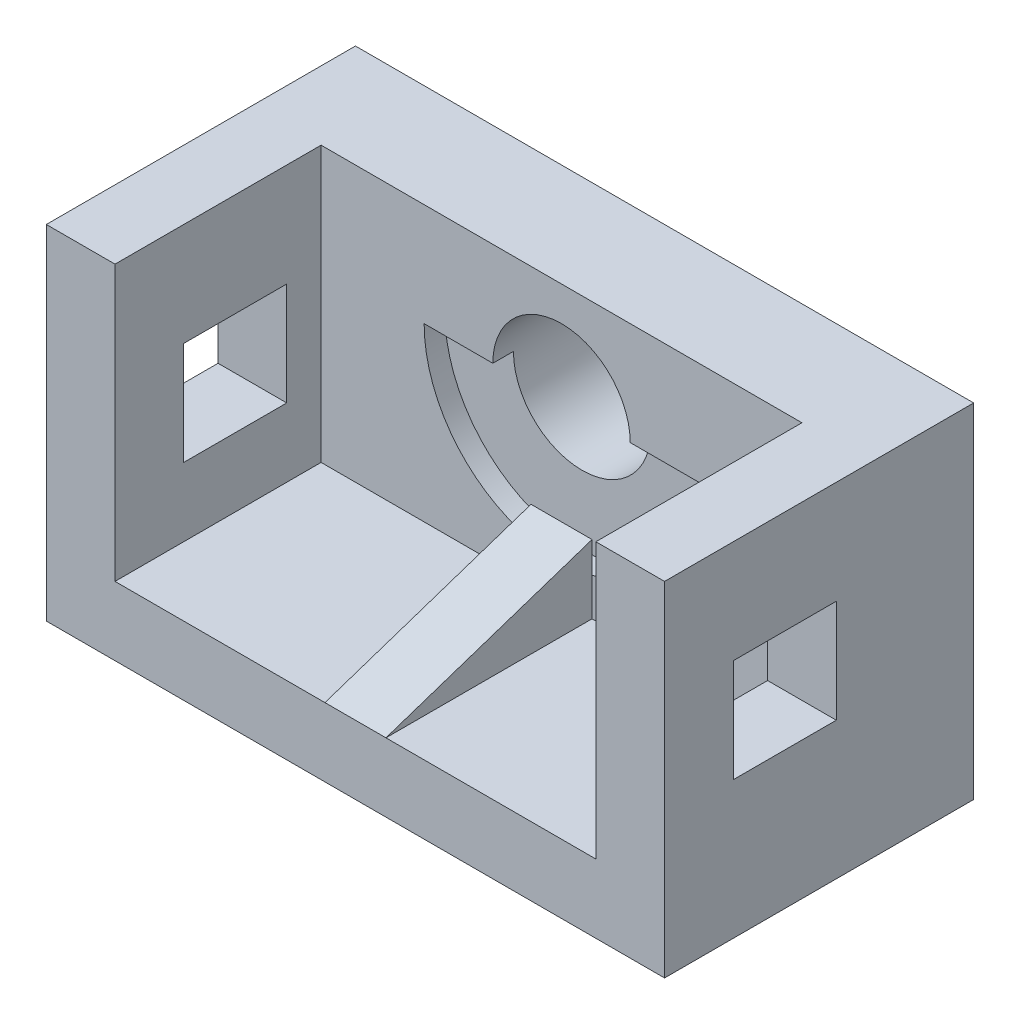
ISO-10303-21;
HEADER;
FILE_DESCRIPTION(('STEP AP214'),'2;1');
FILE_NAME('part.step','',(''),(''),'','','');
FILE_SCHEMA(('AUTOMOTIVE_DESIGN { 1 0 10303 214 1 1 1 1 }'));
ENDSEC;
DATA;
#1=APPLICATION_CONTEXT('core data for automotive mechanical design processes');
#2=APPLICATION_PROTOCOL_DEFINITION('international standard','automotive_design',2000,#1);
#3=PRODUCT_CONTEXT('',#1,'mechanical');
#4=PRODUCT('Part','Part','',(#3));
#5=PRODUCT_RELATED_PRODUCT_CATEGORY('part','',(#4));
#6=PRODUCT_DEFINITION_FORMATION('','',#4);
#7=PRODUCT_DEFINITION_CONTEXT('part definition',#1,'design');
#8=PRODUCT_DEFINITION('design','',#6,#7);
#9=PRODUCT_DEFINITION_SHAPE('','',#8);
#10=(LENGTH_UNIT() NAMED_UNIT(*) SI_UNIT(.MILLI.,.METRE.));
#11=(NAMED_UNIT(*) PLANE_ANGLE_UNIT() SI_UNIT($,.RADIAN.));
#12=(NAMED_UNIT(*) SI_UNIT($,.STERADIAN.) SOLID_ANGLE_UNIT());
#13=UNCERTAINTY_MEASURE_WITH_UNIT(LENGTH_MEASURE(1.E-05),#10,'distance_accuracy_value','');
#14=(GEOMETRIC_REPRESENTATION_CONTEXT(3) GLOBAL_UNCERTAINTY_ASSIGNED_CONTEXT((#13)) GLOBAL_UNIT_ASSIGNED_CONTEXT((#10,
#11,#12)) REPRESENTATION_CONTEXT('',''));
#15=CARTESIAN_POINT('',(0.,0.,0.));
#16=DIRECTION('',(0.,0.,1.));
#17=DIRECTION('',(1.,0.,0.));
#18=AXIS2_PLACEMENT_3D('',#15,#16,#17);
#19=CARTESIAN_POINT('',(-35.,-15.,-30.));
#20=DIRECTION('',(0.,-1.,0.));
#21=DIRECTION('',(0.,0.,-1.));
#22=AXIS2_PLACEMENT_3D('',#19,#20,#21);
#23=PLANE('',#22);
#24=DIRECTION('',(0.,0.,-1.));
#25=VECTOR('',#24,1.);
#26=CARTESIAN_POINT('',(-4.44066466837967,-15.,0.));
#27=LINE('',#26,#25);
#28=CARTESIAN_POINT('',(-4.44066466837967,-15.,0.));
#29=VERTEX_POINT('',#28);
#30=CARTESIAN_POINT('',(-4.44066466837967,-15.,-30.));
#31=VERTEX_POINT('',#30);
#32=EDGE_CURVE('E229',#29,#31,#27,.T.);
#33=ORIENTED_EDGE('',*,*,#32,.T.);
#34=DIRECTION('',(1.,0.,0.));
#35=VECTOR('',#34,1.);
#36=CARTESIAN_POINT('',(-35.,-15.,-30.));
#37=LINE('',#36,#35);
#38=CARTESIAN_POINT('',(-35.,-15.,-30.));
#39=VERTEX_POINT('',#38);
#40=EDGE_CURVE('E350',#39,#31,#37,.T.);
#41=ORIENTED_EDGE('',*,*,#40,.F.);
#42=DIRECTION('',(0.,0.,1.));
#43=VECTOR('',#42,1.);
#44=CARTESIAN_POINT('',(-35.,-15.,-30.));
#45=LINE('',#44,#43);
#46=CARTESIAN_POINT('',(-35.,-15.,0.));
#47=VERTEX_POINT('',#46);
#48=EDGE_CURVE('E254',#39,#47,#45,.T.);
#49=ORIENTED_EDGE('',*,*,#48,.T.);
#50=DIRECTION('',(1.,0.,0.));
#51=VECTOR('',#50,1.);
#52=CARTESIAN_POINT('',(-35.,-15.,0.));
#53=LINE('',#52,#51);
#54=EDGE_CURVE('E240',#47,#29,#53,.T.);
#55=ORIENTED_EDGE('',*,*,#54,.T.);
#56=EDGE_LOOP('',(#33,#41,#49,#55));
#57=FACE_BOUND('',#56,.T.);
#58=ADVANCED_FACE('F39',(#57),#23,.F.);
#59=DIRECTION('',(0.,0.,-1.));
#60=VECTOR('',#59,1.);
#61=CARTESIAN_POINT('',(4.44066466837967,-15.,0.));
#62=LINE('',#61,#60);
#63=CARTESIAN_POINT('',(4.44066466837967,-15.,0.));
#64=VERTEX_POINT('',#63);
#65=CARTESIAN_POINT('',(4.44066466837967,-15.,-30.));
#66=VERTEX_POINT('',#65);
#67=EDGE_CURVE('E218',#64,#66,#62,.T.);
#68=ORIENTED_EDGE('',*,*,#67,.F.);
#69=CARTESIAN_POINT('',(35.,-15.,0.));
#70=VERTEX_POINT('',#69);
#71=EDGE_CURVE('E227',#64,#70,#53,.T.);
#72=ORIENTED_EDGE('',*,*,#71,.T.);
#73=DIRECTION('',(0.,0.,1.));
#74=VECTOR('',#73,1.);
#75=CARTESIAN_POINT('',(35.,-15.,-30.));
#76=LINE('',#75,#74);
#77=CARTESIAN_POINT('',(35.,-15.,-30.));
#78=VERTEX_POINT('',#77);
#79=EDGE_CURVE('E252',#78,#70,#76,.T.);
#80=ORIENTED_EDGE('',*,*,#79,.F.);
#81=EDGE_CURVE('E230',#66,#78,#37,.T.);
#82=ORIENTED_EDGE('',*,*,#81,.F.);
#83=EDGE_LOOP('',(#68,#72,#80,#82));
#84=FACE_BOUND('',#83,.T.);
#85=ADVANCED_FACE('F222',(#84),#23,.F.);
#86=CARTESIAN_POINT('',(0.,0.,-30.));
#87=DIRECTION('',(0.,0.,1.));
#88=DIRECTION('',(1.,0.,0.));
#89=AXIS2_PLACEMENT_3D('',#86,#87,#88);
#90=PLANE('',#89);
#91=CARTESIAN_POINT('',(0.,10.,-30.));
#92=DIRECTION('',(0.,0.,1.));
#93=DIRECTION('',(1.,0.,0.));
#94=AXIS2_PLACEMENT_3D('',#91,#92,#93);
#95=CIRCLE('',#94,20.);
#96=CARTESIAN_POINT('',(-20.,10.,-30.));
#97=VERTEX_POINT('',#96);
#98=CARTESIAN_POINT('',(-4.44066466837967,-9.50078196644956,-30.));
#99=VERTEX_POINT('',#98);
#100=EDGE_CURVE('E371',#97,#99,#95,.T.);
#101=ORIENTED_EDGE('',*,*,#100,.F.);
#102=DIRECTION('',(-1.,0.,0.));
#103=VECTOR('',#102,1.);
#104=CARTESIAN_POINT('',(-10.,10.,-30.));
#105=LINE('',#104,#103);
#106=CARTESIAN_POINT('',(-10.,10.,-30.));
#107=VERTEX_POINT('',#106);
#108=EDGE_CURVE('E678',#107,#97,#105,.T.);
#109=ORIENTED_EDGE('',*,*,#108,.F.);
#110=CARTESIAN_POINT('',(0.,10.,-30.));
#111=DIRECTION('',(0.,0.,1.));
#112=DIRECTION('',(1.,0.,0.));
#113=AXIS2_PLACEMENT_3D('',#110,#111,#112);
#114=CIRCLE('',#113,10.);
#115=CARTESIAN_POINT('',(10.,10.,-30.));
#116=VERTEX_POINT('',#115);
#117=EDGE_CURVE('E336',#116,#107,#114,.T.);
#118=ORIENTED_EDGE('',*,*,#117,.F.);
#119=DIRECTION('',(-1.,0.,0.));
#120=VECTOR('',#119,1.);
#121=CARTESIAN_POINT('',(20.,10.,-30.));
#122=LINE('',#121,#120);
#123=CARTESIAN_POINT('',(20.,10.,-30.));
#124=VERTEX_POINT('',#123);
#125=EDGE_CURVE('E672',#124,#116,#122,.T.);
#126=ORIENTED_EDGE('',*,*,#125,.F.);
#127=CARTESIAN_POINT('',(4.44066466837967,-9.50078196644956,-30.));
#128=VERTEX_POINT('',#127);
#129=EDGE_CURVE('E668',#128,#124,#95,.T.);
#130=ORIENTED_EDGE('',*,*,#129,.F.);
#131=DIRECTION('',(0.,1.,0.));
#132=VECTOR('',#131,1.);
#133=CARTESIAN_POINT('',(4.44066466837967,-5.,-30.));
#134=LINE('',#133,#132);
#135=EDGE_CURVE('E377',#66,#128,#134,.T.);
#136=ORIENTED_EDGE('',*,*,#135,.F.);
#137=ORIENTED_EDGE('',*,*,#81,.T.);
#138=DIRECTION('',(0.,1.,0.));
#139=VECTOR('',#138,1.);
#140=CARTESIAN_POINT('',(35.,-15.,-30.));
#141=LINE('',#140,#139);
#142=CARTESIAN_POINT('',(35.,25.,-30.));
#143=VERTEX_POINT('',#142);
#144=EDGE_CURVE('E260',#78,#143,#141,.T.);
#145=ORIENTED_EDGE('',*,*,#144,.T.);
#146=DIRECTION('',(-1.,0.,0.));
#147=VECTOR('',#146,1.);
#148=CARTESIAN_POINT('',(35.,25.,-30.));
#149=LINE('',#148,#147);
#150=CARTESIAN_POINT('',(-35.,25.,-30.));
#151=VERTEX_POINT('',#150);
#152=EDGE_CURVE('E246',#143,#151,#149,.T.);
#153=ORIENTED_EDGE('',*,*,#152,.T.);
#154=DIRECTION('',(0.,-1.,0.));
#155=VECTOR('',#154,1.);
#156=CARTESIAN_POINT('',(-35.,25.,-30.));
#157=LINE('',#156,#155);
#158=EDGE_CURVE('E343',#151,#39,#157,.T.);
#159=ORIENTED_EDGE('',*,*,#158,.T.);
#160=ORIENTED_EDGE('',*,*,#40,.T.);
#161=DIRECTION('',(0.,-1.,0.));
#162=VECTOR('',#161,1.);
#163=CARTESIAN_POINT('',(-4.44066466837967,-5.,-30.));
#164=LINE('',#163,#162);
#165=EDGE_CURVE('E370',#99,#31,#164,.T.);
#166=ORIENTED_EDGE('',*,*,#165,.F.);
#167=EDGE_LOOP('',(#101,#109,#118,#126,#130,#136,#137,#145,#153,#159,#160,#166));
#168=FACE_BOUND('',#167,.T.);
#169=ADVANCED_FACE('F352',(#168),#90,.T.);
#170=CARTESIAN_POINT('',(45.,25.,-45.));
#171=DIRECTION('',(1.,0.,0.));
#172=DIRECTION('',(0.,0.,-1.));
#173=AXIS2_PLACEMENT_3D('',#170,#171,#172);
#174=PLANE('',#173);
#175=DIRECTION('',(0.,0.,1.));
#176=VECTOR('',#175,1.);
#177=CARTESIAN_POINT('',(45.,-5.,-10.));
#178=LINE('',#177,#176);
#179=CARTESIAN_POINT('',(45.,-5.,-25.));
#180=VERTEX_POINT('',#179);
#181=CARTESIAN_POINT('',(45.,-5.,-10.));
#182=VERTEX_POINT('',#181);
#183=EDGE_CURVE('E383',#180,#182,#178,.T.);
#184=ORIENTED_EDGE('',*,*,#183,.T.);
#185=DIRECTION('',(0.,1.,0.));
#186=VECTOR('',#185,1.);
#187=CARTESIAN_POINT('',(45.,10.,-10.));
#188=LINE('',#187,#186);
#189=CARTESIAN_POINT('',(45.,10.,-10.));
#190=VERTEX_POINT('',#189);
#191=EDGE_CURVE('E389',#182,#190,#188,.T.);
#192=ORIENTED_EDGE('',*,*,#191,.T.);
#193=DIRECTION('',(0.,0.,-1.));
#194=VECTOR('',#193,1.);
#195=CARTESIAN_POINT('',(45.,10.,-25.));
#196=LINE('',#195,#194);
#197=CARTESIAN_POINT('',(45.,10.,-25.));
#198=VERTEX_POINT('',#197);
#199=EDGE_CURVE('E53',#190,#198,#196,.T.);
#200=ORIENTED_EDGE('',*,*,#199,.T.);
#201=DIRECTION('',(0.,-1.,0.));
#202=VECTOR('',#201,1.);
#203=CARTESIAN_POINT('',(45.,-5.,-25.));
#204=LINE('',#203,#202);
#205=EDGE_CURVE('E395',#198,#180,#204,.T.);
#206=ORIENTED_EDGE('',*,*,#205,.T.);
#207=EDGE_LOOP('',(#184,#192,#200,#206));
#208=FACE_BOUND('',#207,.T.);
#209=DIRECTION('',(0.,1.,0.));
#210=VECTOR('',#209,1.);
#211=CARTESIAN_POINT('',(45.,25.,0.));
#212=LINE('',#211,#210);
#213=CARTESIAN_POINT('',(45.,-25.,0.));
#214=VERTEX_POINT('',#213);
#215=CARTESIAN_POINT('',(45.,25.,0.));
#216=VERTEX_POINT('',#215);
#217=EDGE_CURVE('E249',#214,#216,#212,.T.);
#218=ORIENTED_EDGE('',*,*,#217,.F.);
#219=DIRECTION('',(0.,0.,1.));
#220=VECTOR('',#219,1.);
#221=CARTESIAN_POINT('',(45.,-25.,-45.));
#222=LINE('',#221,#220);
#223=CARTESIAN_POINT('',(45.,-25.,-45.));
#224=VERTEX_POINT('',#223);
#225=EDGE_CURVE('E281',#224,#214,#222,.T.);
#226=ORIENTED_EDGE('',*,*,#225,.F.);
#227=DIRECTION('',(0.,1.,0.));
#228=VECTOR('',#227,1.);
#229=CARTESIAN_POINT('',(45.,25.,-45.));
#230=LINE('',#229,#228);
#231=CARTESIAN_POINT('',(45.,25.,-45.));
#232=VERTEX_POINT('',#231);
#233=EDGE_CURVE('E259',#224,#232,#230,.T.);
#234=ORIENTED_EDGE('',*,*,#233,.T.);
#235=DIRECTION('',(0.,0.,1.));
#236=VECTOR('',#235,1.);
#237=CARTESIAN_POINT('',(45.,25.,-45.));
#238=LINE('',#237,#236);
#239=EDGE_CURVE('E272',#232,#216,#238,.T.);
#240=ORIENTED_EDGE('',*,*,#239,.T.);
#241=EDGE_LOOP('',(#218,#226,#234,#240));
#242=FACE_BOUND('',#241,.T.);
#243=ADVANCED_FACE('F41',(#208,#242),#174,.T.);
#244=CARTESIAN_POINT('',(-45.,-25.,-45.));
#245=DIRECTION('',(0.,-1.,0.));
#246=DIRECTION('',(0.,0.,-1.));
#247=AXIS2_PLACEMENT_3D('',#244,#245,#246);
#248=PLANE('',#247);
#249=DIRECTION('',(1.,0.,0.));
#250=VECTOR('',#249,1.);
#251=CARTESIAN_POINT('',(-45.,-25.,0.));
#252=LINE('',#251,#250);
#253=CARTESIAN_POINT('',(-45.,-25.,0.));
#254=VERTEX_POINT('',#253);
#255=EDGE_CURVE('E261',#254,#214,#252,.T.);
#256=ORIENTED_EDGE('',*,*,#255,.F.);
#257=DIRECTION('',(0.,0.,1.));
#258=VECTOR('',#257,1.);
#259=CARTESIAN_POINT('',(-45.,-25.,-45.));
#260=LINE('',#259,#258);
#261=CARTESIAN_POINT('',(-45.,-25.,-45.));
#262=VERTEX_POINT('',#261);
#263=EDGE_CURVE('E282',#262,#254,#260,.T.);
#264=ORIENTED_EDGE('',*,*,#263,.F.);
#265=DIRECTION('',(1.,0.,0.));
#266=VECTOR('',#265,1.);
#267=CARTESIAN_POINT('',(-45.,-25.,-45.));
#268=LINE('',#267,#266);
#269=EDGE_CURVE('E270',#262,#224,#268,.T.);
#270=ORIENTED_EDGE('',*,*,#269,.T.);
#271=ORIENTED_EDGE('',*,*,#225,.T.);
#272=EDGE_LOOP('',(#256,#264,#270,#271));
#273=FACE_BOUND('',#272,.T.);
#274=ADVANCED_FACE('F425',(#273),#248,.T.);
#275=CARTESIAN_POINT('',(-45.,25.,-45.));
#276=DIRECTION('',(-1.,0.,0.));
#277=DIRECTION('',(0.,0.,1.));
#278=AXIS2_PLACEMENT_3D('',#275,#276,#277);
#279=PLANE('',#278);
#280=DIRECTION('',(0.,0.,1.));
#281=VECTOR('',#280,1.);
#282=CARTESIAN_POINT('',(-45.,-5.,-10.));
#283=LINE('',#282,#281);
#284=CARTESIAN_POINT('',(-45.,-5.,-25.));
#285=VERTEX_POINT('',#284);
#286=CARTESIAN_POINT('',(-45.,-5.,-10.));
#287=VERTEX_POINT('',#286);
#288=EDGE_CURVE('E65',#285,#287,#283,.T.);
#289=ORIENTED_EDGE('',*,*,#288,.F.);
#290=DIRECTION('',(0.,-1.,0.));
#291=VECTOR('',#290,1.);
#292=CARTESIAN_POINT('',(-45.,-5.,-25.));
#293=LINE('',#292,#291);
#294=CARTESIAN_POINT('',(-45.,10.,-25.));
#295=VERTEX_POINT('',#294);
#296=EDGE_CURVE('E386',#295,#285,#293,.T.);
#297=ORIENTED_EDGE('',*,*,#296,.F.);
#298=DIRECTION('',(0.,0.,-1.));
#299=VECTOR('',#298,1.);
#300=CARTESIAN_POINT('',(-45.,10.,-25.));
#301=LINE('',#300,#299);
#302=CARTESIAN_POINT('',(-45.,10.,-10.));
#303=VERTEX_POINT('',#302);
#304=EDGE_CURVE('E311',#303,#295,#301,.T.);
#305=ORIENTED_EDGE('',*,*,#304,.F.);
#306=DIRECTION('',(0.,1.,0.));
#307=VECTOR('',#306,1.);
#308=CARTESIAN_POINT('',(-45.,10.,-10.));
#309=LINE('',#308,#307);
#310=EDGE_CURVE('E396',#287,#303,#309,.T.);
#311=ORIENTED_EDGE('',*,*,#310,.F.);
#312=EDGE_LOOP('',(#289,#297,#305,#311));
#313=FACE_BOUND('',#312,.T.);
#314=DIRECTION('',(0.,-1.,0.));
#315=VECTOR('',#314,1.);
#316=CARTESIAN_POINT('',(-45.,25.,0.));
#317=LINE('',#316,#315);
#318=CARTESIAN_POINT('',(-45.,25.,0.));
#319=VERTEX_POINT('',#318);
#320=EDGE_CURVE('E280',#319,#254,#317,.T.);
#321=ORIENTED_EDGE('',*,*,#320,.F.);
#322=DIRECTION('',(0.,0.,1.));
#323=VECTOR('',#322,1.);
#324=CARTESIAN_POINT('',(-45.,25.,-45.));
#325=LINE('',#324,#323);
#326=CARTESIAN_POINT('',(-45.,25.,-45.));
#327=VERTEX_POINT('',#326);
#328=EDGE_CURVE('E286',#327,#319,#325,.T.);
#329=ORIENTED_EDGE('',*,*,#328,.F.);
#330=DIRECTION('',(0.,-1.,0.));
#331=VECTOR('',#330,1.);
#332=CARTESIAN_POINT('',(-45.,25.,-45.));
#333=LINE('',#332,#331);
#334=EDGE_CURVE('E262',#327,#262,#333,.T.);
#335=ORIENTED_EDGE('',*,*,#334,.T.);
#336=ORIENTED_EDGE('',*,*,#263,.T.);
#337=EDGE_LOOP('',(#321,#329,#335,#336));
#338=FACE_BOUND('',#337,.T.);
#339=ADVANCED_FACE('F405',(#313,#338),#279,.T.);
#340=CARTESIAN_POINT('',(-45.,25.,-45.));
#341=DIRECTION('',(0.,1.,0.));
#342=DIRECTION('',(-1.,0.,0.));
#343=AXIS2_PLACEMENT_3D('',#340,#341,#342);
#344=PLANE('',#343);
#345=DIRECTION('',(0.,0.,1.));
#346=VECTOR('',#345,1.);
#347=CARTESIAN_POINT('',(35.,25.,-30.));
#348=LINE('',#347,#346);
#349=CARTESIAN_POINT('',(35.,25.,0.));
#350=VERTEX_POINT('',#349);
#351=EDGE_CURVE('E250',#143,#350,#348,.T.);
#352=ORIENTED_EDGE('',*,*,#351,.T.);
#353=DIRECTION('',(-1.,0.,0.));
#354=VECTOR('',#353,1.);
#355=CARTESIAN_POINT('',(-45.,25.,0.));
#356=LINE('',#355,#354);
#357=EDGE_CURVE('E273',#216,#350,#356,.T.);
#358=ORIENTED_EDGE('',*,*,#357,.F.);
#359=ORIENTED_EDGE('',*,*,#239,.F.);
#360=DIRECTION('',(-1.,0.,0.));
#361=VECTOR('',#360,1.);
#362=CARTESIAN_POINT('',(-45.,25.,-45.));
#363=LINE('',#362,#361);
#364=EDGE_CURVE('E264',#232,#327,#363,.T.);
#365=ORIENTED_EDGE('',*,*,#364,.T.);
#366=ORIENTED_EDGE('',*,*,#328,.T.);
#367=CARTESIAN_POINT('',(-35.,25.,0.));
#368=VERTEX_POINT('',#367);
#369=EDGE_CURVE('E274',#368,#319,#356,.T.);
#370=ORIENTED_EDGE('',*,*,#369,.F.);
#371=DIRECTION('',(0.,0.,1.));
#372=VECTOR('',#371,1.);
#373=CARTESIAN_POINT('',(-35.,25.,-30.));
#374=LINE('',#373,#372);
#375=EDGE_CURVE('E253',#151,#368,#374,.T.);
#376=ORIENTED_EDGE('',*,*,#375,.F.);
#377=ORIENTED_EDGE('',*,*,#152,.F.);
#378=EDGE_LOOP('',(#352,#358,#359,#365,#366,#370,#376,#377));
#379=FACE_BOUND('',#378,.T.);
#380=ADVANCED_FACE('F360',(#379),#344,.T.);
#381=CARTESIAN_POINT('',(0.,0.,-45.));
#382=DIRECTION('',(0.,0.,1.));
#383=DIRECTION('',(1.,0.,0.));
#384=AXIS2_PLACEMENT_3D('',#381,#382,#383);
#385=PLANE('',#384);
#386=CARTESIAN_POINT('',(0.,10.,-45.));
#387=DIRECTION('',(0.,0.,1.));
#388=DIRECTION('',(1.,0.,0.));
#389=AXIS2_PLACEMENT_3D('',#386,#387,#388);
#390=CIRCLE('',#389,10.);
#391=CARTESIAN_POINT('',(10.,10.,-45.));
#392=VERTEX_POINT('',#391);
#393=EDGE_CURVE('E241',#392,#392,#390,.T.);
#394=ORIENTED_EDGE('',*,*,#393,.T.);
#395=EDGE_LOOP('',(#394));
#396=FACE_BOUND('',#395,.T.);
#397=ORIENTED_EDGE('',*,*,#233,.F.);
#398=ORIENTED_EDGE('',*,*,#269,.F.);
#399=ORIENTED_EDGE('',*,*,#334,.F.);
#400=ORIENTED_EDGE('',*,*,#364,.F.);
#401=EDGE_LOOP('',(#397,#398,#399,#400));
#402=FACE_BOUND('',#401,.T.);
#403=ADVANCED_FACE('F433',(#396,#402),#385,.F.);
#404=CARTESIAN_POINT('',(0.,0.,0.));
#405=DIRECTION('',(0.,0.,1.));
#406=DIRECTION('',(1.,0.,0.));
#407=AXIS2_PLACEMENT_3D('',#404,#405,#406);
#408=PLANE('',#407);
#409=DIRECTION('',(1.,0.,0.));
#410=VECTOR('',#409,1.);
#411=CARTESIAN_POINT('',(-5.55933533162033,-15.,0.));
#412=LINE('',#411,#410);
#413=EDGE_CURVE('E201',#29,#64,#412,.T.);
#414=ORIENTED_EDGE('',*,*,#413,.F.);
#415=ORIENTED_EDGE('',*,*,#54,.F.);
#416=DIRECTION('',(0.,-1.,0.));
#417=VECTOR('',#416,1.);
#418=CARTESIAN_POINT('',(-35.,25.,0.));
#419=LINE('',#418,#417);
#420=EDGE_CURVE('E238',#368,#47,#419,.T.);
#421=ORIENTED_EDGE('',*,*,#420,.F.);
#422=ORIENTED_EDGE('',*,*,#369,.T.);
#423=ORIENTED_EDGE('',*,*,#320,.T.);
#424=ORIENTED_EDGE('',*,*,#255,.T.);
#425=ORIENTED_EDGE('',*,*,#217,.T.);
#426=ORIENTED_EDGE('',*,*,#357,.T.);
#427=DIRECTION('',(0.,1.,0.));
#428=VECTOR('',#427,1.);
#429=CARTESIAN_POINT('',(35.,-15.,0.));
#430=LINE('',#429,#428);
#431=EDGE_CURVE('E236',#70,#350,#430,.T.);
#432=ORIENTED_EDGE('',*,*,#431,.F.);
#433=ORIENTED_EDGE('',*,*,#71,.F.);
#434=EDGE_LOOP('',(#414,#415,#421,#422,#423,#424,#425,#426,#432,#433));
#435=FACE_BOUND('',#434,.T.);
#436=ADVANCED_FACE('F234',(#435),#408,.T.);
#437=CARTESIAN_POINT('',(35.,-15.,-30.));
#438=DIRECTION('',(1.,0.,0.));
#439=DIRECTION('',(0.,1.,0.));
#440=AXIS2_PLACEMENT_3D('',#437,#438,#439);
#441=PLANE('',#440);
#442=DIRECTION('',(0.,-1.,0.));
#443=VECTOR('',#442,1.);
#444=CARTESIAN_POINT('',(35.,-15.,-10.));
#445=LINE('',#444,#443);
#446=CARTESIAN_POINT('',(35.,10.,-10.));
#447=VERTEX_POINT('',#446);
#448=CARTESIAN_POINT('',(35.,-5.,-10.));
#449=VERTEX_POINT('',#448);
#450=EDGE_CURVE('E329',#447,#449,#445,.T.);
#451=ORIENTED_EDGE('',*,*,#450,.T.);
#452=DIRECTION('',(0.,0.,-1.));
#453=VECTOR('',#452,1.);
#454=CARTESIAN_POINT('',(35.,-5.,-30.));
#455=LINE('',#454,#453);
#456=CARTESIAN_POINT('',(35.,-5.,-25.));
#457=VERTEX_POINT('',#456);
#458=EDGE_CURVE('E332',#449,#457,#455,.T.);
#459=ORIENTED_EDGE('',*,*,#458,.T.);
#460=DIRECTION('',(0.,1.,0.));
#461=VECTOR('',#460,1.);
#462=CARTESIAN_POINT('',(35.,-15.,-25.));
#463=LINE('',#462,#461);
#464=CARTESIAN_POINT('',(35.,10.,-25.));
#465=VERTEX_POINT('',#464);
#466=EDGE_CURVE('E331',#457,#465,#463,.T.);
#467=ORIENTED_EDGE('',*,*,#466,.T.);
#468=DIRECTION('',(0.,0.,1.));
#469=VECTOR('',#468,1.);
#470=CARTESIAN_POINT('',(35.,10.,-30.));
#471=LINE('',#470,#469);
#472=EDGE_CURVE('E328',#465,#447,#471,.T.);
#473=ORIENTED_EDGE('',*,*,#472,.T.);
#474=EDGE_LOOP('',(#451,#459,#467,#473));
#475=FACE_BOUND('',#474,.T.);
#476=ORIENTED_EDGE('',*,*,#431,.T.);
#477=ORIENTED_EDGE('',*,*,#351,.F.);
#478=ORIENTED_EDGE('',*,*,#144,.F.);
#479=ORIENTED_EDGE('',*,*,#79,.T.);
#480=EDGE_LOOP('',(#476,#477,#478,#479));
#481=FACE_BOUND('',#480,.T.);
#482=ADVANCED_FACE('F412',(#475,#481),#441,.F.);
#483=CARTESIAN_POINT('',(-35.,25.,-30.));
#484=DIRECTION('',(-1.,0.,0.));
#485=DIRECTION('',(0.,-1.,0.));
#486=AXIS2_PLACEMENT_3D('',#483,#484,#485);
#487=PLANE('',#486);
#488=DIRECTION('',(0.,-1.,0.));
#489=VECTOR('',#488,1.);
#490=CARTESIAN_POINT('',(-35.,25.,-25.));
#491=LINE('',#490,#489);
#492=CARTESIAN_POINT('',(-35.,10.,-25.));
#493=VERTEX_POINT('',#492);
#494=CARTESIAN_POINT('',(-35.,-5.,-25.));
#495=VERTEX_POINT('',#494);
#496=EDGE_CURVE('E50',#493,#495,#491,.T.);
#497=ORIENTED_EDGE('',*,*,#496,.T.);
#498=DIRECTION('',(0.,0.,1.));
#499=VECTOR('',#498,1.);
#500=CARTESIAN_POINT('',(-35.,-5.,-30.));
#501=LINE('',#500,#499);
#502=CARTESIAN_POINT('',(-35.,-5.,-10.));
#503=VERTEX_POINT('',#502);
#504=EDGE_CURVE('E11',#495,#503,#501,.T.);
#505=ORIENTED_EDGE('',*,*,#504,.T.);
#506=DIRECTION('',(0.,1.,0.));
#507=VECTOR('',#506,1.);
#508=CARTESIAN_POINT('',(-35.,25.,-10.));
#509=LINE('',#508,#507);
#510=CARTESIAN_POINT('',(-35.,10.,-10.));
#511=VERTEX_POINT('',#510);
#512=EDGE_CURVE('E283',#503,#511,#509,.T.);
#513=ORIENTED_EDGE('',*,*,#512,.T.);
#514=DIRECTION('',(0.,0.,-1.));
#515=VECTOR('',#514,1.);
#516=CARTESIAN_POINT('',(-35.,10.,-30.));
#517=LINE('',#516,#515);
#518=EDGE_CURVE('E291',#511,#493,#517,.T.);
#519=ORIENTED_EDGE('',*,*,#518,.T.);
#520=EDGE_LOOP('',(#497,#505,#513,#519));
#521=FACE_BOUND('',#520,.T.);
#522=ORIENTED_EDGE('',*,*,#420,.T.);
#523=ORIENTED_EDGE('',*,*,#48,.F.);
#524=ORIENTED_EDGE('',*,*,#158,.F.);
#525=ORIENTED_EDGE('',*,*,#375,.T.);
#526=EDGE_LOOP('',(#522,#523,#524,#525));
#527=FACE_BOUND('',#526,.T.);
#528=ADVANCED_FACE('F300',(#521,#527),#487,.F.);
#529=CARTESIAN_POINT('',(0.,10.,-45.));
#530=DIRECTION('',(0.,0.,1.));
#531=DIRECTION('',(1.,0.,0.));
#532=AXIS2_PLACEMENT_3D('',#529,#530,#531);
#533=CYLINDRICAL_SURFACE('',#532,10.);
#534=ORIENTED_EDGE('',*,*,#117,.T.);
#535=DIRECTION('',(0.,0.,1.));
#536=VECTOR('',#535,1.);
#537=CARTESIAN_POINT('',(-10.,10.,-33.));
#538=LINE('',#537,#536);
#539=CARTESIAN_POINT('',(-10.,10.,-33.));
#540=VERTEX_POINT('',#539);
#541=EDGE_CURVE('E688',#540,#107,#538,.T.);
#542=ORIENTED_EDGE('',*,*,#541,.F.);
#543=CARTESIAN_POINT('',(0.,10.,-33.));
#544=DIRECTION('',(0.,0.,-1.));
#545=DIRECTION('',(1.,0.,0.));
#546=AXIS2_PLACEMENT_3D('',#543,#544,#545);
#547=CIRCLE('',#546,10.);
#548=CARTESIAN_POINT('',(10.,10.,-33.));
#549=VERTEX_POINT('',#548);
#550=EDGE_CURVE('E693',#549,#540,#547,.T.);
#551=ORIENTED_EDGE('',*,*,#550,.F.);
#552=DIRECTION('',(0.,0.,1.));
#553=VECTOR('',#552,1.);
#554=CARTESIAN_POINT('',(10.,10.,-33.));
#555=LINE('',#554,#553);
#556=EDGE_CURVE('E686',#549,#116,#555,.T.);
#557=ORIENTED_EDGE('',*,*,#556,.T.);
#558=EDGE_LOOP('',(#534,#542,#551,#557));
#559=FACE_BOUND('',#558,.T.);
#560=ORIENTED_EDGE('',*,*,#393,.F.);
#561=EDGE_LOOP('',(#560));
#562=FACE_BOUND('',#561,.T.);
#563=ADVANCED_FACE('F451',(#559,#562),#533,.F.);
#564=CARTESIAN_POINT('',(45.,10.,-10.));
#565=DIRECTION('',(0.,0.,1.));
#566=DIRECTION('',(1.,0.,0.));
#567=AXIS2_PLACEMENT_3D('',#564,#565,#566);
#568=PLANE('',#567);
#569=DIRECTION('',(-1.,0.,0.));
#570=VECTOR('',#569,1.);
#571=CARTESIAN_POINT('',(45.,-5.,-10.));
#572=LINE('',#571,#570);
#573=EDGE_CURVE('E323',#503,#287,#572,.T.);
#574=ORIENTED_EDGE('',*,*,#573,.T.);
#575=ORIENTED_EDGE('',*,*,#310,.T.);
#576=DIRECTION('',(-1.,0.,0.));
#577=VECTOR('',#576,1.);
#578=CARTESIAN_POINT('',(45.,10.,-10.));
#579=LINE('',#578,#577);
#580=EDGE_CURVE('E320',#511,#303,#579,.T.);
#581=ORIENTED_EDGE('',*,*,#580,.F.);
#582=ORIENTED_EDGE('',*,*,#512,.F.);
#583=EDGE_LOOP('',(#574,#575,#581,#582));
#584=FACE_BOUND('',#583,.T.);
#585=ADVANCED_FACE('F403',(#584),#568,.F.);
#586=CARTESIAN_POINT('',(45.,10.,-25.));
#587=DIRECTION('',(0.,1.,0.));
#588=DIRECTION('',(0.,0.,1.));
#589=AXIS2_PLACEMENT_3D('',#586,#587,#588);
#590=PLANE('',#589);
#591=ORIENTED_EDGE('',*,*,#580,.T.);
#592=ORIENTED_EDGE('',*,*,#304,.T.);
#593=DIRECTION('',(-1.,0.,0.));
#594=VECTOR('',#593,1.);
#595=CARTESIAN_POINT('',(45.,10.,-25.));
#596=LINE('',#595,#594);
#597=EDGE_CURVE('E304',#493,#295,#596,.T.);
#598=ORIENTED_EDGE('',*,*,#597,.F.);
#599=ORIENTED_EDGE('',*,*,#518,.F.);
#600=EDGE_LOOP('',(#591,#592,#598,#599));
#601=FACE_BOUND('',#600,.T.);
#602=ADVANCED_FACE('F307',(#601),#590,.F.);
#603=CARTESIAN_POINT('',(45.,-5.,-25.));
#604=DIRECTION('',(0.,0.,-1.));
#605=DIRECTION('',(-1.,0.,0.));
#606=AXIS2_PLACEMENT_3D('',#603,#604,#605);
#607=PLANE('',#606);
#608=ORIENTED_EDGE('',*,*,#597,.T.);
#609=ORIENTED_EDGE('',*,*,#296,.T.);
#610=DIRECTION('',(-1.,0.,0.));
#611=VECTOR('',#610,1.);
#612=CARTESIAN_POINT('',(45.,-5.,-25.));
#613=LINE('',#612,#611);
#614=EDGE_CURVE('E310',#495,#285,#613,.T.);
#615=ORIENTED_EDGE('',*,*,#614,.F.);
#616=ORIENTED_EDGE('',*,*,#496,.F.);
#617=EDGE_LOOP('',(#608,#609,#615,#616));
#618=FACE_BOUND('',#617,.T.);
#619=ADVANCED_FACE('F303',(#618),#607,.F.);
#620=CARTESIAN_POINT('',(45.,-5.,-10.));
#621=DIRECTION('',(0.,-1.,0.));
#622=DIRECTION('',(0.,0.,-1.));
#623=AXIS2_PLACEMENT_3D('',#620,#621,#622);
#624=PLANE('',#623);
#625=ORIENTED_EDGE('',*,*,#614,.T.);
#626=ORIENTED_EDGE('',*,*,#288,.T.);
#627=ORIENTED_EDGE('',*,*,#573,.F.);
#628=ORIENTED_EDGE('',*,*,#504,.F.);
#629=EDGE_LOOP('',(#625,#626,#627,#628));
#630=FACE_BOUND('',#629,.T.);
#631=ADVANCED_FACE('F407',(#630),#624,.F.);
#632=EDGE_CURVE('E324',#182,#449,#572,.T.);
#633=ORIENTED_EDGE('',*,*,#632,.F.);
#634=ORIENTED_EDGE('',*,*,#183,.F.);
#635=EDGE_CURVE('E318',#180,#457,#613,.T.);
#636=ORIENTED_EDGE('',*,*,#635,.T.);
#637=ORIENTED_EDGE('',*,*,#458,.F.);
#638=EDGE_LOOP('',(#633,#634,#636,#637));
#639=FACE_BOUND('',#638,.T.);
#640=ADVANCED_FACE('F414',(#639),#624,.F.);
#641=ORIENTED_EDGE('',*,*,#635,.F.);
#642=ORIENTED_EDGE('',*,*,#205,.F.);
#643=EDGE_CURVE('E312',#198,#465,#596,.T.);
#644=ORIENTED_EDGE('',*,*,#643,.T.);
#645=ORIENTED_EDGE('',*,*,#466,.F.);
#646=EDGE_LOOP('',(#641,#642,#644,#645));
#647=FACE_BOUND('',#646,.T.);
#648=ADVANCED_FACE('F417',(#647),#607,.F.);
#649=ORIENTED_EDGE('',*,*,#643,.F.);
#650=ORIENTED_EDGE('',*,*,#199,.F.);
#651=EDGE_CURVE('E313',#190,#447,#579,.T.);
#652=ORIENTED_EDGE('',*,*,#651,.T.);
#653=ORIENTED_EDGE('',*,*,#472,.F.);
#654=EDGE_LOOP('',(#649,#650,#652,#653));
#655=FACE_BOUND('',#654,.T.);
#656=ADVANCED_FACE('F418',(#655),#590,.F.);
#657=ORIENTED_EDGE('',*,*,#651,.F.);
#658=ORIENTED_EDGE('',*,*,#191,.F.);
#659=ORIENTED_EDGE('',*,*,#632,.T.);
#660=ORIENTED_EDGE('',*,*,#450,.F.);
#661=EDGE_LOOP('',(#657,#658,#659,#660));
#662=FACE_BOUND('',#661,.T.);
#663=ADVANCED_FACE('F416',(#662),#568,.F.);
#664=CARTESIAN_POINT('',(-4.44066466837967,-5.,0.));
#665=DIRECTION('',(1.,0.,0.));
#666=DIRECTION('',(0.,1.,0.));
#667=AXIS2_PLACEMENT_3D('',#664,#665,#666);
#668=PLANE('',#667);
#669=ORIENTED_EDGE('',*,*,#32,.F.);
#670=DIRECTION('',(0.,0.316227766016838,-0.948683298050514));
#671=VECTOR('',#670,1.);
#672=CARTESIAN_POINT('',(-4.44066466837967,-14.,-3.));
#673=LINE('',#672,#671);
#674=CARTESIAN_POINT('',(-4.44066466837967,-5.,-30.));
#675=VERTEX_POINT('',#674);
#676=EDGE_CURVE('E206',#29,#675,#673,.T.);
#677=ORIENTED_EDGE('',*,*,#676,.T.);
#678=EDGE_CURVE('E373',#675,#99,#164,.T.);
#679=ORIENTED_EDGE('',*,*,#678,.T.);
#680=ORIENTED_EDGE('',*,*,#165,.T.);
#681=EDGE_LOOP('',(#669,#677,#679,#680));
#682=FACE_BOUND('',#681,.T.);
#683=ADVANCED_FACE('F376',(#682),#668,.F.);
#684=CARTESIAN_POINT('',(4.44066466837967,-5.,0.));
#685=DIRECTION('',(-1.,0.,0.));
#686=DIRECTION('',(0.,-1.,0.));
#687=AXIS2_PLACEMENT_3D('',#684,#685,#686);
#688=PLANE('',#687);
#689=DIRECTION('',(0.,1.,0.));
#690=VECTOR('',#689,1.);
#691=CARTESIAN_POINT('',(4.44066466837967,-5.,-30.));
#692=LINE('',#691,#690);
#693=CARTESIAN_POINT('',(4.44066466837967,-5.,-30.));
#694=VERTEX_POINT('',#693);
#695=EDGE_CURVE('E224',#128,#694,#692,.T.);
#696=ORIENTED_EDGE('',*,*,#695,.T.);
#697=DIRECTION('',(0.,0.316227766016838,-0.948683298050514));
#698=VECTOR('',#697,1.);
#699=CARTESIAN_POINT('',(4.44066466837967,-15.,0.));
#700=LINE('',#699,#698);
#701=EDGE_CURVE('E202',#64,#694,#700,.T.);
#702=ORIENTED_EDGE('',*,*,#701,.F.);
#703=ORIENTED_EDGE('',*,*,#67,.T.);
#704=ORIENTED_EDGE('',*,*,#135,.T.);
#705=EDGE_LOOP('',(#696,#702,#703,#704));
#706=FACE_BOUND('',#705,.T.);
#707=ADVANCED_FACE('F216',(#706),#688,.F.);
#708=CARTESIAN_POINT('',(0.,10.,-30.));
#709=DIRECTION('',(0.,0.,1.));
#710=DIRECTION('',(1.,0.,0.));
#711=AXIS2_PLACEMENT_3D('',#708,#709,#710);
#712=PLANE('',#711);
#713=DIRECTION('',(-1.,0.,0.));
#714=VECTOR('',#713,1.);
#715=CARTESIAN_POINT('',(4.44066466837967,-5.,-30.));
#716=LINE('',#715,#714);
#717=EDGE_CURVE('E233',#694,#675,#716,.T.);
#718=ORIENTED_EDGE('',*,*,#717,.F.);
#719=ORIENTED_EDGE('',*,*,#695,.F.);
#720=EDGE_CURVE('E670',#99,#128,#95,.T.);
#721=ORIENTED_EDGE('',*,*,#720,.F.);
#722=ORIENTED_EDGE('',*,*,#678,.F.);
#723=EDGE_LOOP('',(#718,#719,#721,#722));
#724=FACE_BOUND('',#723,.T.);
#725=ADVANCED_FACE('F542',(#724),#712,.F.);
#726=CARTESIAN_POINT('',(0.,10.,-33.));
#727=DIRECTION('',(0.,0.,1.));
#728=DIRECTION('',(1.,0.,0.));
#729=AXIS2_PLACEMENT_3D('',#726,#727,#728);
#730=CYLINDRICAL_SURFACE('',#729,20.);
#731=ORIENTED_EDGE('',*,*,#100,.T.);
#732=ORIENTED_EDGE('',*,*,#720,.T.);
#733=ORIENTED_EDGE('',*,*,#129,.T.);
#734=DIRECTION('',(0.,0.,1.));
#735=VECTOR('',#734,1.);
#736=CARTESIAN_POINT('',(20.,10.,-33.));
#737=LINE('',#736,#735);
#738=CARTESIAN_POINT('',(20.,10.,-33.));
#739=VERTEX_POINT('',#738);
#740=EDGE_CURVE('E689',#739,#124,#737,.T.);
#741=ORIENTED_EDGE('',*,*,#740,.F.);
#742=CARTESIAN_POINT('',(0.,10.,-33.));
#743=DIRECTION('',(0.,0.,1.));
#744=DIRECTION('',(1.,0.,0.));
#745=AXIS2_PLACEMENT_3D('',#742,#743,#744);
#746=CIRCLE('',#745,20.);
#747=CARTESIAN_POINT('',(-20.,10.,-33.));
#748=VERTEX_POINT('',#747);
#749=EDGE_CURVE('E682',#748,#739,#746,.T.);
#750=ORIENTED_EDGE('',*,*,#749,.F.);
#751=DIRECTION('',(0.,0.,1.));
#752=VECTOR('',#751,1.);
#753=CARTESIAN_POINT('',(-20.,10.,-33.));
#754=LINE('',#753,#752);
#755=EDGE_CURVE('E669',#748,#97,#754,.T.);
#756=ORIENTED_EDGE('',*,*,#755,.T.);
#757=EDGE_LOOP('',(#731,#732,#733,#741,#750,#756));
#758=FACE_BOUND('',#757,.T.);
#759=ADVANCED_FACE('F538',(#758),#730,.F.);
#760=CARTESIAN_POINT('',(-10.,10.,-33.));
#761=DIRECTION('',(0.,1.,0.));
#762=DIRECTION('',(0.,0.,1.));
#763=AXIS2_PLACEMENT_3D('',#760,#761,#762);
#764=PLANE('',#763);
#765=ORIENTED_EDGE('',*,*,#108,.T.);
#766=ORIENTED_EDGE('',*,*,#755,.F.);
#767=DIRECTION('',(-1.,0.,0.));
#768=VECTOR('',#767,1.);
#769=CARTESIAN_POINT('',(-10.,10.,-33.));
#770=LINE('',#769,#768);
#771=EDGE_CURVE('E687',#540,#748,#770,.T.);
#772=ORIENTED_EDGE('',*,*,#771,.F.);
#773=ORIENTED_EDGE('',*,*,#541,.T.);
#774=EDGE_LOOP('',(#765,#766,#772,#773));
#775=FACE_BOUND('',#774,.T.);
#776=ADVANCED_FACE('F543',(#775),#764,.F.);
#777=CARTESIAN_POINT('',(20.,10.,-33.));
#778=DIRECTION('',(0.,1.,0.));
#779=DIRECTION('',(0.,0.,1.));
#780=AXIS2_PLACEMENT_3D('',#777,#778,#779);
#781=PLANE('',#780);
#782=ORIENTED_EDGE('',*,*,#125,.T.);
#783=ORIENTED_EDGE('',*,*,#556,.F.);
#784=DIRECTION('',(-1.,0.,0.));
#785=VECTOR('',#784,1.);
#786=CARTESIAN_POINT('',(20.,10.,-33.));
#787=LINE('',#786,#785);
#788=EDGE_CURVE('E696',#739,#549,#787,.T.);
#789=ORIENTED_EDGE('',*,*,#788,.F.);
#790=ORIENTED_EDGE('',*,*,#740,.T.);
#791=EDGE_LOOP('',(#782,#783,#789,#790));
#792=FACE_BOUND('',#791,.T.);
#793=ADVANCED_FACE('F554',(#792),#781,.F.);
#794=CARTESIAN_POINT('',(0.,10.,-33.));
#795=DIRECTION('',(0.,0.,1.));
#796=DIRECTION('',(1.,0.,0.));
#797=AXIS2_PLACEMENT_3D('',#794,#795,#796);
#798=PLANE('',#797);
#799=ORIENTED_EDGE('',*,*,#749,.T.);
#800=ORIENTED_EDGE('',*,*,#788,.T.);
#801=ORIENTED_EDGE('',*,*,#550,.T.);
#802=ORIENTED_EDGE('',*,*,#771,.T.);
#803=EDGE_LOOP('',(#799,#800,#801,#802));
#804=FACE_BOUND('',#803,.T.);
#805=ADVANCED_FACE('F563',(#804),#798,.T.);
#806=CARTESIAN_POINT('',(-5.55933533162033,-15.,0.));
#807=DIRECTION('',(0.,-0.948683298050514,-0.316227766016838));
#808=DIRECTION('',(0.,0.316227766016838,-0.948683298050514));
#809=AXIS2_PLACEMENT_3D('',#806,#807,#808);
#810=PLANE('',#809);
#811=ORIENTED_EDGE('',*,*,#413,.T.);
#812=ORIENTED_EDGE('',*,*,#701,.T.);
#813=ORIENTED_EDGE('',*,*,#717,.T.);
#814=ORIENTED_EDGE('',*,*,#676,.F.);
#815=EDGE_LOOP('',(#811,#812,#813,#814));
#816=FACE_BOUND('',#815,.T.);
#817=ADVANCED_FACE('F203',(#816),#810,.F.);
#818=CLOSED_SHELL('',(#58,#85,#169,#243,#274,#339,#380,#403,#436,#482,#528,#563,#585,#602,#619,
#631,#640,#648,#656,#663,#683,#707,#725,#759,#776,#793,#805,#817));
#819=MANIFOLD_SOLID_BREP('B2',#818);
#820=ADVANCED_BREP_SHAPE_REPRESENTATION('',(#18,#819),#14);
#821=SHAPE_DEFINITION_REPRESENTATION(#9,#820);
ENDSEC;
END-ISO-10303-21;
